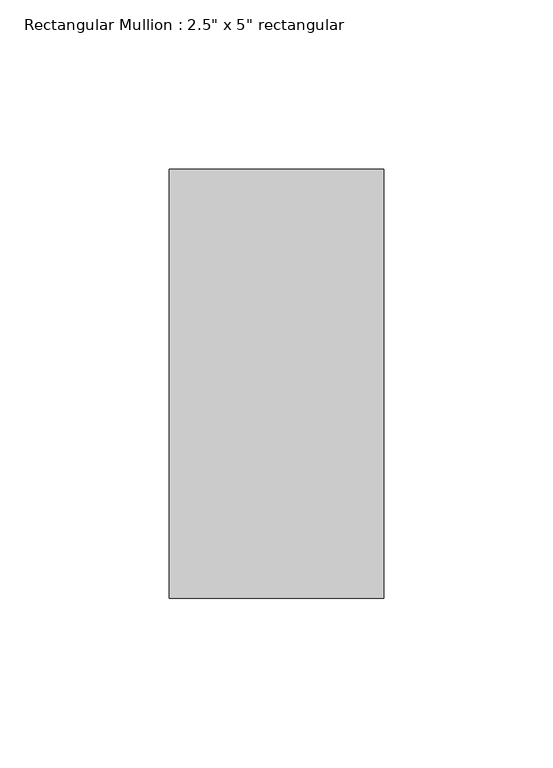
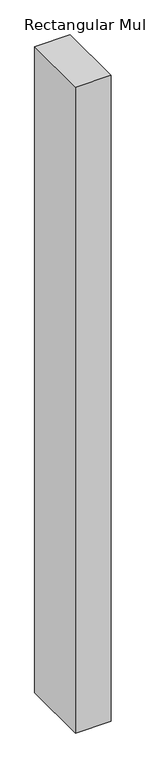
"""IFC4 building model written with IfcOpenShell, lengths in millimetres: member geometry."""

from ifc_helpers import new_model, si_unit, frame, origin, place, context, project, spatial, polyline, outline, extrude, source, transform, mapped, element, save


def member_9771a04b(model_context):
    return source(origin(), model_context, "Body", "SweptSolid", [
        extrude(outline(polyline([(0.0, 63.5), (0.0, -63.5), (-63.5, -63.5), (-63.5, 63.5), (0.0, 63.5)])), frame((0.0, 0.0, -1225.55), z_axis=(0.0, 0.0, 1.0), x_axis=(1.0, 0.0, 0.0)), (0.0, 0.0, 1.0), 1225.55),
    ])


if __name__ == "__main__":
    model = new_model("IFC4")
    model_context = context("Model", 3, world=origin())
    ifc_project = project(units=[si_unit("LENGTHUNIT", "METRE", prefix="MILLI")], contexts=[model_context])
    site = spatial("IfcSite", under=ifc_project)
    building = spatial("IfcBuilding", under=site)
    placement = place(None, origin())
    member_shape = member_9771a04b(model_context)
    element("IfcMember", 1, ObjectType="Rectangular Mullion : 2.5\" x 5\" rectangular", at=placement, inside=building, context=model_context, shape_type="MappedRepresentation", body=[
        mapped(member_shape, transform((0.0, 0.0, 0.0), x_axis=(1.0, 0.0, 0.0), y_axis=(0.0, 1.0, 0.0), z_axis=(0.0, 0.0, 1.0))),
    ])
    save(model, "model.ifc")

# Revit data of these elements
# Type "Rectangular Mullion : 2.5\" x 5\" rectangular"
#   built-in parameter 1007304 = 0.416667 (stored number, unit not read)
#   built-in parameter 1007301 = 0.104167 (stored number, unit not read)
#   built-in parameter 1007300 = 0.104167 (stored number, unit not read)
# Element 1 (IfcMember, "Rectangular Mullion : 2.5\" x 5\" rectangular")
#   Materials on its faces: "Iron, Ductile"
# Materials
#   "Iron, Ductile": class "Metal", colour RGB 0 0 0, transparency 0, Description = "Ductile cast iron", Cost = 0
